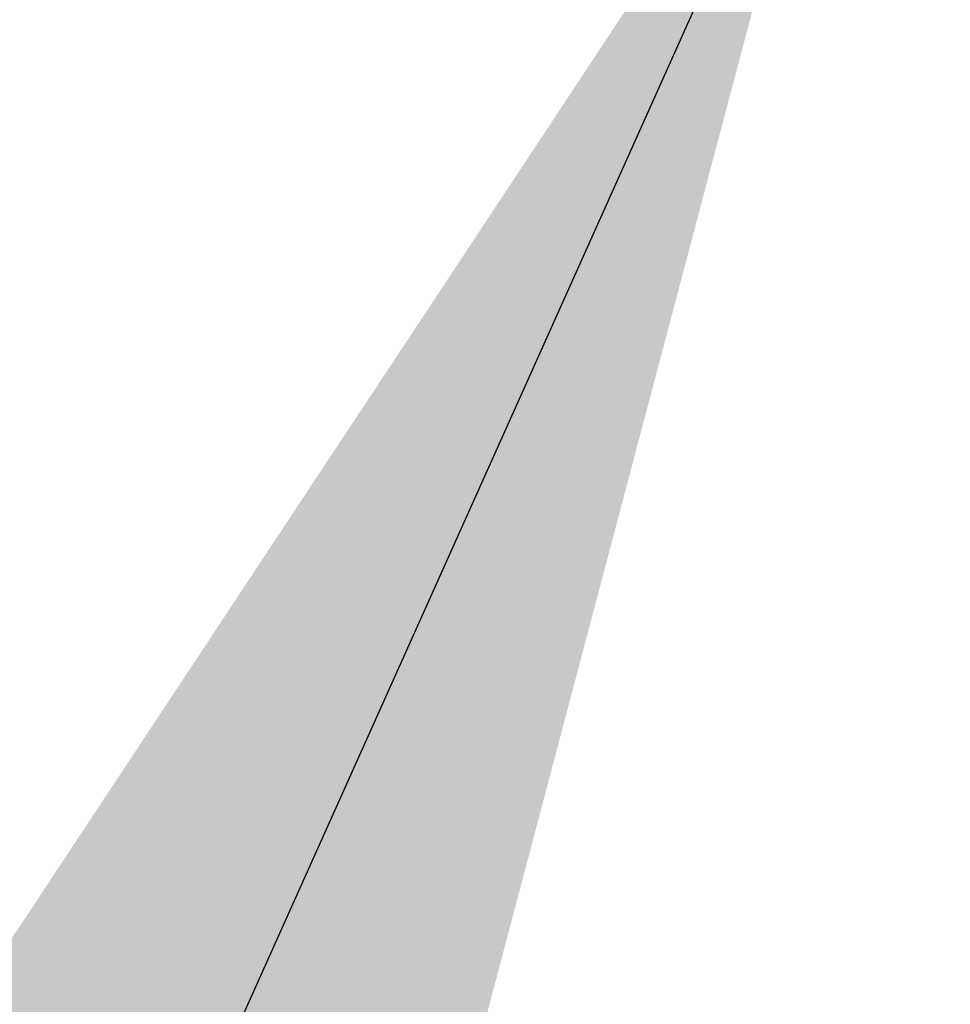
# Model space of a CAD drawing. Units: inches. Extents: x -9413 to 9703, y -9719 to 9096.
# Tile 1 of 1: x -0.3 to 275.6, y -311.2 to -19.4. Entities that reach past the tile are written whole.
import ezdxf
from ezdxf import colors
from ezdxf.entities.mleader import LeaderData, LeaderLine
from ezdxf.math import Vec2, Vec3

# ---------------------------------------------------------------- set-up
doc = ezdxf.new("R2010")
doc.units = ezdxf.units.IN
doc.header["$MEASUREMENT"] = 0
doc.layers.add('M-ANNO-TEXT', color=7, linetype='Continuous', lineweight=18)
doc.styles.get("Standard").update_dxf_attribs({"font": 'arial.ttf'})

msp = doc.modelspace()

# ---------------------------------------------------------------- leaders
at = {"layer": 'M-ANNO-TEXT'}
ml = msp.add_multileader_mtext('Standard', dxfattribs=at)
ml.set_content('Air preheater', color=256)
ml.set_leader_properties()
ml.build(insert=Vec2(0, 0))
ml.multileader.update_dxf_attribs({"dogleg_length": 0.36, "arrow_head_size": 10000, "scale": 10})
ctx = ml.context
ctx.base_point, ctx.scale, ctx.char_height, ctx.arrow_head_size, ctx.landing_gap_size, ctx.plane_origin = Vec3(229.7079293124727, 37.30650895205824), 10, 5.4, 10000, 0.9, Vec3(241.9833706008503, 78.04556948044049)
notes = []
notes.append((ctx, [(1, (1, 1, 0), (223.7048975654645, 37.30650895205824), (1, 0), 6.003031747008185, [(0, [(241.9833706008503, 78.04556948044049)], 0, [])])]))
ctx.mtext.insert, ctx.mtext.flow_direction = Vec3(230.6079293124727, 40.75609967511417), 5
for ctx, leaders in notes:
    for number, flags, end, landing, length, lines in leaders:
        leader = LeaderData()
        leader.index, (leader.has_last_leader_line, leader.has_dogleg_vector, leader.attachment_direction) = number, flags
        leader.last_leader_point, leader.dogleg_vector, leader.dogleg_length = Vec3(end), Vec3(landing), length
        for number, points, colour, breaks in lines:
            line = LeaderLine()
            line.index, line.vertices, line.color, line.breaks = number, Vec3.list(points), colors.encode_raw_color(colour), breaks
            leader.lines.append(line)
        ctx.leaders.append(leader)

doc.saveas('drawing.dxf')
